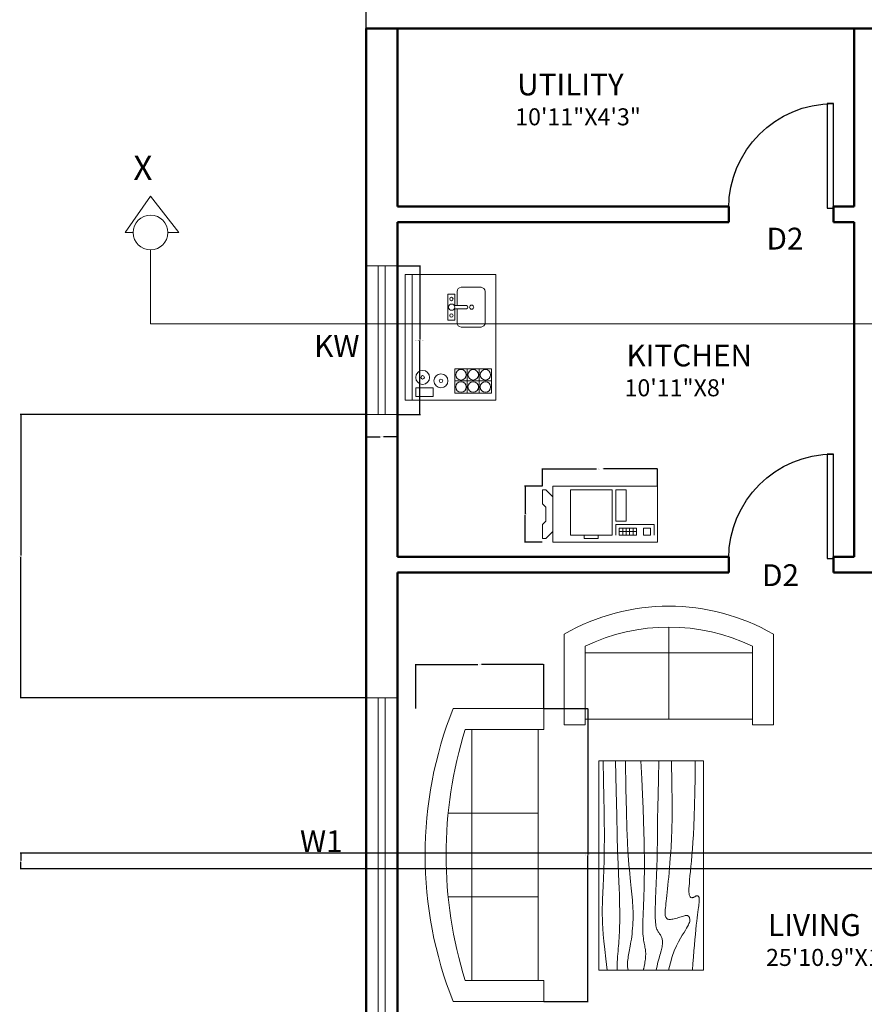
# Model space of a CAD drawing. Units: inches. Extents: x 7359 to 7979, y 33027 to 34263.
# Tile 5 of 32: x 7369 to 7612, y 33347 to 33630. Entities that reach past the tile are written whole.
import ezdxf

# ---------------------------------------------------------------- set-up
doc = ezdxf.new("R2010")
doc.units = ezdxf.units.IN
for name, color, linetype, lineweight in [('A-ANNO-DIMS', 2, 'Continuous', 18), ('A-ANNO-SYMB', 7, 'Continuous', 18), ('A-ANNO-TEXT', 3, 'Continuous', 18), ('A-AREA-IDEN', 7, 'Continuous', 18), ('A-DOOR', 3, 'Continuous', 25), ('A-EQPM', 8, 'Continuous', 18), ('A-FLOR-FIXT', 9, 'Continuous', 18), ('A-FURN', 8, 'Continuous', 18), ('A-GLAZ', 4, 'Continuous', 18), ('A-WALL', 7, 'Continuous', 50)]:
    doc.layers.add(name, color=color, linetype=linetype, lineweight=lineweight)
doc.styles.get("Standard").update_dxf_attribs({"font": 'arial.ttf'})
doc.dimstyles.get("Standard").update_dxf_attribs({"dimtxt": 0.18, "dimasz": 0.18, "dimexe": 0.18, "dimexo": 0.0625, "dimgap": 0.09, "dimtad": 0, "dimtih": 1, "dimtoh": 1, "dimdec": 4, "dimzin": 0, "dimdsep": 46, "dimtxsty": 'Standard', "dimcen": 0.09, "dimadec": 0, "dimazin": 0, "dimtfac": 1, "dimtdec": 4, "dimtofl": 0, "dimtmove": 0, "dimatfit": 3, "dimfxl": 1, "dimtolj": 1, "dimtzin": 0, "dimarcsym": 0})

# ---------------------------------------------------------------- blocks, each defined once
blk = doc.blocks.new('*U2')
for p, q in [((0, 0), (0, -100)), ((750, 0), (750, -100))]:
    blk.add_line(p, q)
blk.add_lwpolyline([(0, 0), (0, 750), (43.75, 750), (43.75, 0)], close=True)
blk.add_arc((0, 0), 750, 0, 90)
blk = doc.blocks.new('Table - Rectangular Woodgrain 60 x 30 in.')
for p, q in [((0, 0), (0, -30)), ((60, 0), (0, 0)), ((60, -30), (60, 0)), ((0, -30), (60, -30))]:
    blk.add_line(p, q)
for points in [[(0, -2.4), (4.8155, -2.418), (9.0302, -2.4688), (12.709, -2.5477), (15.9167, -2.65), (18.7181, -2.7711), (21.1781, -2.9063), (23.3616, -3.0508), (25.3333, -3.2), (27.1477, -3.3495), (28.8172, -3.4958), (30.3437, -3.636), (31.7291, -3.7667), (32.9756, -3.8849), (34.0849, -3.9875), (35.059, -4.0714), (35.9, -4.1334), (36.6114, -4.1711), (37.2041, -4.1854), (37.6906, -4.1779), (38.0833, -4.15), (38.3948, -4.1034), (38.6375, -4.0396), (38.8239, -3.9602), (38.9666, -3.8667), (39.0764, -3.7608), (39.1573, -3.6448), (39.2116, -3.521), (39.2416, -3.3917), (39.2498, -3.2593), (39.2385, -3.1261), (39.21, -2.9944), (39.1666, -2.8667), (39.111, -2.7447), (39.0468, -2.6281), (38.978, -2.5163), (38.9083, -2.4083), (38.8418, -2.3035), (38.7823, -2.201), (38.7337, -2.1001), (38.7, -2), (38.6844, -1.9003), (38.6875, -1.8021), (38.7094, -1.707), (38.75, -1.6167), (38.8094, -1.5326), (38.8875, -1.4563), (38.9844, -1.3893), (39.1, -1.3333), (39.2351, -1.2896), (39.3937, -1.2583), (39.5804, -1.2396), (39.8, -1.2333), (40.057, -1.2396), (40.3562, -1.2583), (40.7023, -1.2896), (41.1, -1.3333), (41.5547, -1.3895), (42.0755, -1.4573), (42.6721, -1.5361), (43.3542, -1.625), (44.1316, -1.7233), (45.014, -1.8302), (46.0114, -1.9449), (47.1333, -2.0667), (48.3862, -2.1947), (49.7625, -2.3281), (51.2513, -2.4663), (52.8416, -2.6083), (54.5226, -2.7535), (56.2833, -2.9011), (58.1127, -3.0501), (60, -3.2)], [(0, -9.2), (6.5759, -9.0858), (11.9385, -9.0365), (16.2527, -9.0418), (19.6833, -9.0917), (22.3952, -9.1759), (24.5531, -9.2844), (26.322, -9.4069), (27.8666, -9.5333), (29.3241, -9.6553), (30.7203, -9.7719), (32.0532, -9.8837), (33.3208, -9.9917), (34.5213, -10.0965), (35.6526, -10.199), (36.7128, -10.2999), (37.7, -10.4), (38.6129, -10.4996), (39.4531, -10.5969), (40.223, -10.6895), (40.925, -10.775), (41.5613, -10.8512), (42.1344, -10.9156), (42.6465, -10.966), (43.1, -11), (43.4976, -11.0158), (43.8437, -11.0136), (44.143, -10.9942), (44.4, -10.9583), (44.6195, -10.9069), (44.8062, -10.8406), (44.9648, -10.7603), (45.1, -10.6667), (45.2155, -10.5598), (45.3114, -10.4365), (45.3871, -10.2929), (45.4416, -10.125), (45.4743, -9.929), (45.4844, -9.7011), (45.4709, -9.4371), (45.4333, -9.1333), (45.3716, -8.7883), (45.2896, -8.4104), (45.1919, -8.0107), (45.0833, -7.6), (44.9685, -7.1893), (44.8521, -6.7896), (44.7388, -6.4117), (44.6333, -6.0667), (44.54, -5.7628), (44.4614, -5.4979), (44.4001, -5.2675), (44.3583, -5.0667), (44.3384, -4.8909), (44.3427, -4.7354), (44.3736, -4.5956), (44.4333, -4.4667), (44.5236, -4.3453), (44.6427, -4.2333), (44.7884, -4.1339), (44.9583, -4.05), (45.1501, -3.9849), (45.3614, -3.9417), (45.59, -3.9234), (45.8333, -3.9333), (46.0915, -3.9749), (46.3734, -4.0531), (46.6906, -4.1736), (47.0542, -4.3417), (47.4756, -4.5629), (47.9661, -4.8427), (48.5372, -5.1866), (49.2, -5.6), (49.9676, -6.0844), (50.8594, -6.625), (51.8965, -7.2031), (53.1, -7.8), (54.491, -8.3969), (56.0906, -8.975), (57.9199, -9.5156), (60, -10)], [(0, -12.8), (5.1847, -12.9322), (9.6213, -13.0323), (13.3963, -13.1059), (16.5958, -13.1583), (19.3063, -13.1952), (21.614, -13.2219), (23.6054, -13.2439), (25.3666, -13.2667), (26.9728, -13.2947), (28.4531, -13.3281), (29.8256, -13.3663), (31.1083, -13.4083), (32.3191, -13.4535), (33.476, -13.501), (34.597, -13.5501), (35.7, -13.6), (36.7984, -13.6497), (37.8875, -13.6979), (38.9578, -13.743), (40, -13.7833), (41.0047, -13.8174), (41.9625, -13.8438), (42.864, -13.8607), (43.7, -13.8667), (44.4631, -13.8604), (45.1552, -13.8417), (45.7801, -13.8104), (46.3416, -13.7667), (46.8439, -13.7104), (47.2906, -13.6417), (47.6858, -13.5604), (48.0333, -13.4667), (48.3375, -13.3608), (48.6042, -13.2448), (48.8396, -13.121), (49.05, -12.9917), (49.2417, -12.8593), (49.4208, -12.7261), (49.5937, -12.5944), (49.7667, -12.4667), (49.9452, -12.3451), (50.1323, -12.2313), (50.3303, -12.1268), (50.5416, -12.0333), (50.7686, -11.9524), (51.0135, -11.8854), (51.2788, -11.8341), (51.5666, -11.8), (51.8785, -11.7843), (52.2116, -11.7865), (52.562, -11.8059), (52.926, -11.8417), (53.2998, -11.8931), (53.6795, -11.9594), (54.0614, -12.0397), (54.4416, -12.1333), (54.8223, -12.2401), (55.2293, -12.3625), (55.6942, -12.5037), (56.2489, -12.6667), (56.9251, -12.8547), (57.7545, -13.0708), (58.7689, -13.3182), (60, -13.6)], [(0, -18), (5.124, -17.7273), (9.6609, -17.5057), (13.6705, -17.3303), (17.2125, -17.1958), (20.3467, -17.0973), (23.1328, -17.0297), (25.6307, -16.9878), (27.9, -16.9667), (29.9928, -16.9617), (31.9302, -16.9703), (33.7254, -16.9907), (35.3917, -17.0208), (36.9423, -17.0588), (38.3906, -17.1026), (39.7499, -17.1503), (41.0333, -17.2), (42.2519, -17.2496), (43.4073, -17.2969), (44.4986, -17.3395), (45.525, -17.375), (46.4858, -17.4012), (47.3802, -17.4156), (48.2074, -17.416), (48.9667, -17.4), (49.6583, -17.3662), (50.2872, -17.3167), (50.8595, -17.2547), (51.3812, -17.1833), (51.8584, -17.1057), (52.2971, -17.025), (52.7034, -16.9443), (53.0833, -16.8667), (53.443, -16.7951), (53.789, -16.7313), (54.128, -16.6768), (54.4666, -16.6334), (54.8115, -16.6024), (55.1693, -16.5854), (55.5465, -16.5841), (55.95, -16.6), (56.3828, -16.6337), (56.8346, -16.6823), (57.2915, -16.7418), (57.7396, -16.8084), (58.165, -16.878), (58.5539, -16.9469), (58.8924, -17.0111), (59.1666, -17.0667), (59.3679, -17.1107), (59.5078, -17.1438), (59.6032, -17.1675), (59.6708, -17.1833), (59.7275, -17.193), (59.7901, -17.1979), (59.8753, -17.1998), (60, -17.2)], [(0, -22.4), (8.0098, -22.2501), (14.4094, -22.1011), (19.4168, -21.9535), (23.25, -21.8083), (26.1269, -21.6663), (28.2656, -21.5281), (29.884, -21.3947), (31.2, -21.2667), (32.3967, -21.1448), (33.5172, -21.0292), (34.5697, -20.9198), (35.5625, -20.8167), (36.5037, -20.7198), (37.4015, -20.6292), (38.2642, -20.5448), (39.1, -20.4667), (39.9164, -20.3951), (40.7187, -20.3313), (41.5117, -20.2768), (42.3, -20.2333), (43.0883, -20.2024), (43.8812, -20.1854), (44.6836, -20.1841), (45.5, -20.2), (46.3328, -20.234), (47.1747, -20.2844), (48.0163, -20.3488), (48.8479, -20.425), (49.66, -20.5106), (50.4429, -20.6031), (51.1872, -20.7004), (51.8833, -20.8), (52.5246, -20.8999), (53.1166, -20.9995), (53.6681, -21.0983), (54.1875, -21.1958), (54.6834, -21.2919), (55.1646, -21.3859), (55.6394, -21.4777), (56.1167, -21.5667), (56.6028, -21.6515), (57.0961, -21.7266), (57.5929, -21.7852), (58.0896, -21.8208), (58.5823, -21.8268), (59.0674, -21.7964), (59.5412, -21.723), (60, -21.6)], [(0, -25.2), (8.6355, -25.0504), (15.7026, -24.9031), (21.4049, -24.7606), (25.9458, -24.625), (29.529, -24.4988), (32.3578, -24.3844), (34.6359, -24.284), (36.5667, -24.2), (38.3213, -24.1341), (39.9417, -24.0854), (41.437, -24.0523), (42.8167, -24.0333), (44.0901, -24.0268), (45.2667, -24.0313), (46.3557, -24.0451), (47.3667, -24.0667), (48.309, -24.0947), (49.1928, -24.1287), (50.0284, -24.168), (50.826, -24.2125), (51.5959, -24.2617), (52.3483, -24.3151), (53.0935, -24.3725), (53.8417, -24.4334), (54.6009, -24.497), (55.3699, -24.561), (56.1454, -24.6226), (56.9239, -24.6792), (57.7021, -24.7279), (58.4764, -24.7662), (59.2435, -24.7911), (60, -24.8)], [(0, -28.8), (5.6867, -28.6681), (10.45, -28.5698), (14.407, -28.5012), (17.675, -28.4584), (20.3711, -28.4374), (22.6125, -28.4344), (24.5164, -28.4455), (26.2, -28.4667), (27.762, -28.4947), (29.2276, -28.5281), (30.6033, -28.5663), (31.8958, -28.6084), (33.1118, -28.6535), (34.2578, -28.7011), (35.3405, -28.7501), (36.3666, -28.8), (37.3443, -28.8497), (38.288, -28.8974), (39.2137, -28.9412), (40.1375, -28.9792), (41.0753, -29.0093), (42.0432, -29.0297), (43.0572, -29.0384), (44.1333, -29.0333), (45.2936, -29.0114), (46.5843, -28.9641), (48.0579, -28.8816), (49.7666, -28.7542), (51.7629, -28.5721), (54.0989, -28.3255), (56.8272, -28.0048), (60, -27.6)]]:
    blk.add_lwpolyline(points)
blk = doc.blocks.new('Sofa - Roundback 7 ft.')
for p, q in [((-12.00002, -32.4421), (-12.00003, -6.5971)), ((11.99997, -32.4421), (11.99998, -6.5971)), ((-36.000027, -34), (-36.000027, -11.4696)), ((-35.999844, -13.3819), (35.9998, -13.3819)), ((35.99998, -34), (35.99998, -11.4696)), ((-36.000027, -32.4421), (35.99998, -32.4421))]:
    blk.add_line(p, q)
for points in [[(-36.000027, -34), (-42.000027, -34), (-42.000027, -8)], [(41.99998, -8), (41.99998, -34), (35.99998, -34)]]:
    blk.add_lwpolyline(points)
for centre, radius, start, end in [((0, -114.25), 114.25, 68.43141, 111.5686), ((-0.00001, -127.1968), 121.1968, 72.72033, 107.2797)]:
    blk.add_arc(centre, radius, start, end)
blk = doc.blocks.new('Sofa - Roundback Loveseat 5 ft.')
for p, q in [((0, -32.44198), (0, -5.99998)), ((-24, -33.99998), (-24, -11.46958)), ((-23.9998, -13.38178), (23.99986, -13.38178)), ((24.00004, -33.99998), (24.00004, -11.46958)), ((-24, -32.44198), (24.00004, -32.44198))]:
    blk.add_line(p, q)
for points in [[(-24, -33.99998), (-30, -33.99998), (-30, -7.99998)], [(30.00004, -7.99998), (30.00004, -33.99998), (24.00004, -33.99998)]]:
    blk.add_lwpolyline(points)
for centre, radius, start, end in [((0, -60.24998), 60.24998, 60.13715, 119.8628), ((0, -61.38438), 55.38444, 64.32083, 115.6792)]:
    blk.add_arc(centre, radius, start, end)
blk = doc.blocks.new('Wet Bar')
for p, q in [((0, 0), (36, 0)), ((0, -26), (0, 0)), ((36, 0), (36, -26)), ((0, -2), (36, -2)), ((3.5, -3), (1, -3)), ((1, -3), (1, -8)), ((3.5, -8), (3.5, -3)), ((1, -8), (3.5, -8)), ((2, -14.25), (9, -14.25)), ((2, -24.75), (2, -14.25)), ((5.5, -14.25), (5.5, -24.75)), ((9, -14.25), (9, -24.75)), ((26.2, -17.55), (26.2, -14.1284)), ((27.1001, -17.55), (27.1001, -14.1284)), ((2, -17.75), (9, -17.75)), ((9, -21.25), (2, -21.25)), ((9, -24.75), (2, -24.75)), ((36, -26), (0, -26))]:
    blk.add_line(p, q)
for points in [[(26.2, -14.25), (22.95, -14.25), (22.95, -12.2), (26.75, -12.2)], [(26.7487, -12.2), (30.3501, -12.2), (30.3501, -14.25), (27.1001, -14.25)], [(20.95, -21.75), (20.95, -16.05)], [(22.15, -14.85), (26.2, -14.85)], [(27.1001, -14.85), (31.15, -14.85)], [(32.3501, -16.05), (32.3501, -21.75)], [(31.15, -22.95), (22.15, -22.95)]]:
    blk.add_lwpolyline(points)
for centre, radius in [((6.5, -5), 2), ((6.5, -5), 0.5), ((5.5, -10.25), 2), ((5.5, -10.25), 0.5), ((24.25, -13.25), 0.5), ((26.65, -13.35), 0.9), ((29, -13.25), 0.5), ((3.75, -16), 1.5), ((7.25, -16), 1.5), ((3.75, -19.5), 1.5), ((7.25, -19.5), 1.5), ((26.65, -19.05), 0.6), ((3.75, -23), 1.5), ((7.25, -23), 1.5)]:
    blk.add_circle(centre, radius)
for centre, radius, start, end in [((22.2251, -16.125), 1.2772, 93.36646, 176.6335), ((31.075, -16.125), 1.2772, 3.366461, 86.63354), ((26.65, -17.55), 0.45, 180, 0), ((22.2251, -21.675), 1.2772, 183.3665, 266.6335), ((31.075, -21.675), 1.2772, 273.3665, 356.6335)]:
    blk.add_arc(centre, radius, start, end)
blk = doc.blocks.new('Copy Machine')
for p, q in [((0, 0), (0, -16)), ((30, 0), (0, 0)), ((30, -16), (30, 0)), ((-3, -1), (-3, -5)), ((-2, -1), (-3, -1)), ((0, -3), (-2, -1)), ((5, -1), (5, -14)), ((17, -1), (5, -1)), ((17, -14), (17, -1)), ((18, -1), (18, -10)), ((21, -1), (18, -1)), ((21, -10), (21, -1)), ((-3, -5), (-2, -6)), ((-2, -10), (-2, -6)), ((-3, -11), (-2, -10)), ((-3, -15), (-3, -11)), ((18, -10), (21, -10)), ((18, -14), (18, -11)), ((18, -11), (29, -11)), ((29, -11), (29, -14)), ((0, -13), (-2, -15)), ((5, -14), (17, -14)), ((9, -14), (9, -15)), ((13, -15), (13, -14)), ((24, -12), (19, -12)), ((19, -12), (19, -14)), ((24, -13), (19, -13)), ((19, -14), (24, -14)), ((20, -12), (20, -14)), ((21, -14), (21, -12)), ((22, -12), (22, -14)), ((23, -14), (23, -12)), ((24, -14), (24, -12)), ((28, -12), (26, -12)), ((26, -12), (26, -14)), ((26, -14), (28, -14)), ((28, -14), (28, -12)), ((-2, -15), (-3, -15)), ((0, -16), (30, -16)), ((9, -15), (13, -15))]:
    blk.add_line(p, q)
blk = doc.blocks.new('SECTION-HEAD')
for p, q in [((0, 4.98), (7.32, 15.43)), ((7.32, 15.43), (15.39, 4.98)), ((2.34, 4.98), (0, 4.98)), ((12.3, 4.98), (15.39, 4.98))]:
    blk.add_line(p, q)
blk.add_circle((7.32, 4.98), 4.98)
blk = doc.blocks.new('WINDOW-W1-LIVING')
for p, q in [((0, 91.75), (9, 91.75)), ((3.5, 0), (3.5, 91.75)), ((5.5, 0), (5.5, 91.75)), ((0, 0), (9, 0))]:
    blk.add_line(p, q)
blk = doc.blocks.new('WINDOW-KW')
for p, q in [((0, 42.66), (9, 42.66)), ((3.5, 42.66), (3.5, 0)), ((5.5, 42.66), (5.5, 0)), ((5.5, 42.66), (5.5, 0)), ((0, 0), (9, 0))]:
    blk.add_line(p, q)
blk = doc.blocks.new('*D40')
at = {"layer": 'A-ANNO-DIMS', "color": 0, "lineweight": -2, "transparency": 16777216}
for p, q in [((7519.73, 33432.15), (7532.45, 33432.15)), ((7532.27, 33431.97), (7532.27, 33390.34)), ((7532.27, 33348.33), (7532.27, 33389.97)), ((7519.73, 33348.15), (7532.45, 33348.15))]:
    blk.add_line(p, q, dxfattribs=at)
at = {"layer": 'A-ANNO-DIMS', "color": 0, "transparency": 16777216}
for points in [[(7532.24, 33431.97), (7532.3, 33431.97), (7532.27, 33432.15)], [(7532.24, 33348.33), (7532.3, 33348.33), (7532.27, 33348.15)]]:
    blk.add_solid(points, dxfattribs=at)
at = {"layer": 'Defpoints', "color": 0, "transparency": 16777216}
for p in [(7519.67, 33432.15), (7532.27, 33432.15), (7519.67, 33348.15)]:
    blk.add_point(p, dxfattribs=at)
at = {"layer": 'A-ANNO-DIMS', "color": 0, "transparency": 16777216, "insert": (7532.27, 33390.15), "char_height": 0.18, "attachment_point": 5}
blk.add_mtext('\\A1;SOFA 84 TYP.', dxfattribs=at)
blk = doc.blocks.new('*D41')
at = {"layer": 'A-ANNO-DIMS', "color": 0, "lineweight": -2, "transparency": 16777216}
for p, q in [((7483.01, 33432.22), (7483.01, 33444.93)), ((7483.19, 33444.75), (7500.81, 33444.75)), ((7519.49, 33444.75), (7501.87, 33444.75)), ((7519.67, 33432.22), (7519.67, 33444.93))]:
    blk.add_line(p, q, dxfattribs=at)
at = {"layer": 'A-ANNO-DIMS', "color": 0, "transparency": 16777216}
for points in [[(7483.19, 33444.78), (7483.19, 33444.72), (7483.01, 33444.75)], [(7519.49, 33444.78), (7519.49, 33444.72), (7519.67, 33444.75)]]:
    blk.add_solid(points, dxfattribs=at)
at = {"layer": 'Defpoints', "color": 0, "transparency": 16777216}
for p in [(7483.01, 33444.75), (7483.01, 33432.15), (7519.67, 33432.15)]:
    blk.add_point(p, dxfattribs=at)
at = {"layer": 'A-ANNO-DIMS', "color": 0, "transparency": 16777216, "insert": (7501.34, 33444.75), "char_height": 0.18, "attachment_point": 5}
blk.add_mtext('\\A1;37 TYP.', dxfattribs=at)
blk = doc.blocks.new('*D44')
at = {"layer": 'A-ANNO-DIMS', "color": 0, "lineweight": -2, "transparency": 16777216}
for p, q in [((7519.31, 33495.98), (7519.31, 33501.05)), ((7519.49, 33500.87), (7534.76, 33500.87)), ((7552.13, 33500.87), (7536.85, 33500.87)), ((7552.31, 33495.98), (7552.31, 33501.05))]:
    blk.add_line(p, q, dxfattribs=at)
at = {"layer": 'A-ANNO-DIMS', "color": 0, "transparency": 16777216}
for points in [[(7519.49, 33500.9), (7519.49, 33500.84), (7519.31, 33500.87)], [(7552.13, 33500.9), (7552.13, 33500.84), (7552.31, 33500.87)]]:
    blk.add_solid(points, dxfattribs=at)
at = {"layer": 'Defpoints', "color": 0, "transparency": 16777216}
for p in [(7552.31, 33500.87), (7519.31, 33495.92), (7552.31, 33495.92)]:
    blk.add_point(p, dxfattribs=at)
at = {"layer": 'A-ANNO-DIMS', "color": 0, "transparency": 16777216, "insert": (7535.81, 33500.87), "char_height": 0.18, "attachment_point": 5}
blk.add_mtext('\\A1;COPIER 33 TYP.', dxfattribs=at)
blk = doc.blocks.new('*D45')
at = {"layer": 'A-ANNO-DIMS', "color": 0, "lineweight": -2, "transparency": 16777216}
for p, q in [((7519.25, 33495.92), (7514.18, 33495.92)), ((7514.36, 33495.74), (7514.36, 33488.1)), ((7514.36, 33480.1), (7514.36, 33487.74)), ((7519.25, 33479.92), (7514.18, 33479.92))]:
    blk.add_line(p, q, dxfattribs=at)
at = {"layer": 'A-ANNO-DIMS', "color": 0, "transparency": 16777216}
for points in [[(7514.33, 33495.74), (7514.39, 33495.74), (7514.36, 33495.92)], [(7514.33, 33480.1), (7514.39, 33480.1), (7514.36, 33479.92)]]:
    blk.add_solid(points, dxfattribs=at)
at = {"layer": 'Defpoints', "color": 0, "transparency": 16777216}
for p in [(7514.36, 33495.92), (7519.31, 33495.92), (7519.31, 33479.92)]:
    blk.add_point(p, dxfattribs=at)
at = {"layer": 'A-ANNO-DIMS', "color": 0, "transparency": 16777216, "insert": (7514.36, 33487.92), "char_height": 0.18, "attachment_point": 5}
blk.add_mtext('\\A1;16 TYP.', dxfattribs=at)
blk = doc.blocks.new('*D58')
at = {"layer": 'A-ANNO-DIMS', "color": 0, "lineweight": -2, "transparency": 16777216}
for p, q in [((7477.79, 33559.14), (7484.31, 33559.14)), ((7484.13, 33558.96), (7484.13, 33538)), ((7484.13, 33516.66), (7484.13, 33537.63)), ((7477.79, 33516.48), (7484.31, 33516.48))]:
    blk.add_line(p, q, dxfattribs=at)
at = {"layer": 'A-ANNO-DIMS', "color": 0, "transparency": 16777216}
for points in [[(7484.1, 33558.96), (7484.16, 33558.96), (7484.13, 33559.14)], [(7484.1, 33516.66), (7484.16, 33516.66), (7484.13, 33516.48)]]:
    blk.add_solid(points, dxfattribs=at)
at = {"layer": 'Defpoints', "color": 0, "transparency": 16777216}
for p in [(7477.73, 33559.14), (7484.13, 33559.14), (7477.73, 33516.48)]:
    blk.add_point(p, dxfattribs=at)
at = {"layer": 'A-ANNO-DIMS', "color": 0, "transparency": 16777216, "insert": (7484.13, 33537.81), "char_height": 0.18, "attachment_point": 5}
blk.add_mtext('\\A1;KITCHEN KW 43 TYP.', dxfattribs=at)
blk = doc.blocks.new('*D59')
at = {"layer": 'A-ANNO-DIMS', "color": 0, "lineweight": -2, "transparency": 16777216}
for p, q in [((7468.73, 33516.42), (7468.73, 33509.91)), ((7477.73, 33516.42), (7477.73, 33509.91)), ((7468.91, 33510.09), (7472.77, 33510.09)), ((7477.55, 33510.09), (7473.68, 33510.09))]:
    blk.add_line(p, q, dxfattribs=at)
at = {"layer": 'A-ANNO-DIMS', "color": 0, "transparency": 16777216}
for points in [[(7468.91, 33510.12), (7468.91, 33510.06), (7468.73, 33510.09)], [(7477.55, 33510.12), (7477.55, 33510.06), (7477.73, 33510.09)]]:
    blk.add_solid(points, dxfattribs=at)
at = {"layer": 'Defpoints', "color": 0, "transparency": 16777216}
for p in [(7468.73, 33516.48), (7477.73, 33516.48), (7477.73, 33510.09)]:
    blk.add_point(p, dxfattribs=at)
at = {"layer": 'A-ANNO-DIMS', "color": 0, "transparency": 16777216, "insert": (7473.23, 33510.09), "char_height": 0.18, "attachment_point": 5}
blk.add_mtext('\\A1;9 TYP.', dxfattribs=at)
blk = doc.blocks.new('*D66')
at = {"layer": 'A-ANNO-DIMS', "color": 0, "lineweight": -2, "transparency": 16777216}
for p, q in [((7468.73, 33627.22), (7468.73, 33657.24)), ((7468.91, 33657.06), (7681.03, 33657.06)), ((7893.95, 33657.06), (7681.82, 33657.06)), ((7894.13, 33627.22), (7894.13, 33657.24))]:
    blk.add_line(p, q, dxfattribs=at)
at = {"layer": 'A-ANNO-DIMS', "color": 0, "transparency": 16777216}
for points in [[(7468.91, 33657.09), (7468.91, 33657.03), (7468.73, 33657.06)], [(7893.95, 33657.09), (7893.95, 33657.03), (7894.13, 33657.06)]]:
    blk.add_solid(points, dxfattribs=at)
at = {"layer": 'Defpoints', "color": 0, "transparency": 16777216}
for p in [(7894.13, 33657.06), (7468.73, 33627.16), (7894.13, 33627.16)]:
    blk.add_point(p, dxfattribs=at)
at = {"layer": 'A-ANNO-DIMS', "color": 0, "transparency": 16777216, "insert": (7681.43, 33657.06), "char_height": 0.18, "attachment_point": 5}
blk.add_mtext('\\A1;425.4', dxfattribs=at)
blk = doc.blocks.new('*D81')
at = {"layer": 'A-ANNO-DIMS', "color": 0, "lineweight": -2, "transparency": 16777216}
for p, q in [((7468.66, 33516.48), (7369.54, 33516.48)), ((7369.72, 33516.3), (7369.72, 33476.05)), ((7369.72, 33435.44), (7369.72, 33475.69)), ((7468.66, 33435.26), (7369.54, 33435.26))]:
    blk.add_line(p, q, dxfattribs=at)
at = {"layer": 'A-ANNO-DIMS', "color": 0, "transparency": 16777216}
for points in [[(7369.69, 33516.3), (7369.75, 33516.3), (7369.72, 33516.48)], [(7369.69, 33435.44), (7369.75, 33435.44), (7369.72, 33435.26)]]:
    blk.add_solid(points, dxfattribs=at)
at = {"layer": 'Defpoints', "color": 0, "transparency": 16777216}
for p in [(7369.72, 33516.48), (7468.73, 33516.48), (7468.73, 33435.26)]:
    blk.add_point(p, dxfattribs=at)
at = {"layer": 'A-ANNO-DIMS', "color": 0, "transparency": 16777216, "insert": (7369.72, 33475.87), "char_height": 0.18, "attachment_point": 5}
blk.add_mtext('\\A1;81.22', dxfattribs=at)
blk = doc.blocks.new('*D85')
at = {"layer": 'A-ANNO-DIMS', "color": 0, "lineweight": -2, "transparency": 16777216}
for p, q in [((7793.06, 33390.66), (7369.54, 33390.66)), ((7369.72, 33390.48), (7369.72, 33388.59)), ((7793.06, 33386.16), (7369.54, 33386.16)), ((7369.72, 33386.34), (7369.72, 33388.23))]:
    blk.add_line(p, q, dxfattribs=at)
at = {"layer": 'A-ANNO-DIMS', "color": 0, "transparency": 16777216}
for points in [[(7369.69, 33390.48), (7369.75, 33390.48), (7369.72, 33390.66)], [(7369.69, 33386.34), (7369.75, 33386.34), (7369.72, 33386.16)]]:
    blk.add_solid(points, dxfattribs=at)
at = {"layer": 'Defpoints', "color": 0, "transparency": 16777216}
for p in [(7793.13, 33390.66), (7369.72, 33386.16), (7793.13, 33386.16)]:
    blk.add_point(p, dxfattribs=at)
at = {"layer": 'A-ANNO-DIMS', "color": 0, "transparency": 16777216, "insert": (7369.72, 33388.41), "char_height": 0.18, "attachment_point": 5}
blk.add_mtext('\\A1;4.5', dxfattribs=at)

msp = doc.modelspace()

# ---------------------------------------------------------------- linework, layer by layer
at = {"layer": 'A-ANNO-SYMB'}
for q in [(7406.9423, 33563.6906), (7940.6696, 33542.482)]:
    msp.add_line((7406.9423, 33542.482), q, dxfattribs=at)
at = {"layer": 'A-WALL'}
for p, q in [((7468.7266, 33627.1623), (7894.1266, 33627.1623)), ((7468.7266, 33627.1623), (7468.7266, 33158.6623)), ((7477.7266, 33627.1623), (7477.7266, 33576.1623)), ((7608.7266, 33627.1623), (7608.7266, 33576.1623)), ((7477.7266, 33576.1623), (7572.7266, 33576.1623)), ((7572.7266, 33576.1623), (7572.7266, 33571.6623)), ((7602.7266, 33576.1623), (7608.7266, 33576.1623)), ((7602.7266, 33576.1623), (7602.7266, 33571.6623)), ((7477.7266, 33571.6623), (7572.7266, 33571.6623)), ((7477.7266, 33571.6623), (7477.7266, 33475.6623)), ((7602.7266, 33571.6623), (7608.7266, 33571.6623)), ((7608.7266, 33571.6623), (7608.7266, 33475.6623)), ((7477.7266, 33475.6623), (7572.7266, 33475.6623)), ((7572.7266, 33475.6623), (7572.7266, 33471.1623)), ((7602.7266, 33475.6623), (7608.7266, 33475.6623)), ((7602.7266, 33475.6623), (7602.7266, 33471.1623)), ((7477.7266, 33471.1623), (7572.7266, 33471.1623)), ((7477.7266, 33471.1623), (7477.7266, 33301.0623)), ((7602.7266, 33471.1623), (7691.2266, 33471.1623))]:
    msp.add_line(p, q, dxfattribs=at)

# ---------------------------------------------------------------- block references
at = {"layer": 'A-ANNO-SYMB'}
msp.add_blockref('SECTION-HEAD', (7399.6221, 33563.6904), dxfattribs=at)
at = {"layer": 'A-DOOR', "xscale": -0.0399999999999999, "yscale": 0.0399999999999999, "zscale": 0.0399999999999999}
for p in [(7602.7266, 33575.6623), (7602.7266, 33475.1623)]:
    msp.add_blockref('*U2', p, dxfattribs=at)
at = {"layer": 'A-EQPM'}
msp.add_blockref('Copy Machine', (7522.3083, 33495.9203), dxfattribs=at)
at = {"layer": 'A-FLOR-FIXT', "rotation": 90}
msp.add_blockref('Wet Bar', (7479.9538, 33520.6382), dxfattribs=at)
at = {"layer": 'A-FURN'}
msp.add_blockref('Sofa - Roundback Loveseat 5 ft.', (7555.532, 33461.52), dxfattribs=at)
for name, p, rotation in [('Sofa - Roundback 7 ft.', (7485.6721, 33390.1541), 90), ('Table - Rectangular Woodgrain 60 x 30 in.', (7565.492, 33417.1564), 270)]:
    msp.add_blockref(name, p, dxfattribs=dict(at, rotation=rotation))
at = {"layer": 'A-GLAZ'}
for name, p in [('WINDOW-KW', (7468.7261, 33516.4844)), ('WINDOW-W1-LIVING', (7468.7261, 33343.5154))]:
    msp.add_blockref(name, p, dxfattribs=at)

# ---------------------------------------------------------------- texts
at = {"layer": 'A-ANNO-SYMB'}
msp.add_text('X', height=6.9459, dxfattribs=at).set_placement((7402.022, 33583.7843))
at = {"layer": 'A-ANNO-TEXT'}
for s, p in [('D2', (7583.5367, 33563.809)), ('KW', (7453.831, 33533.0184)), ('D2', (7582.2569, 33467.2804)), ('W1', (7449.7806, 33390.9721))]:
    msp.add_text(s, height=6.25941, dxfattribs=at).set_placement(p)
at = {"layer": 'A-AREA-IDEN'}
for s, height, p in [('UTILITY', 6.25941, (7512.0433, 33608.0303)), ('10\'11"X4\'3"', 4.885549, (7511.48, 33599.4359)), ('KITCHEN', 6.25941, (7543.3947, 33530.309)), ('10\'11"X8\'', 4.88555, (7542.8315, 33521.7147)), ('LIVING', 6.25941, (7583.9722, 33366.9355)), ('25\'10.9"X14\'1.6"', 4.885549, (7583.409, 33358.3411))]:
    msp.add_text(s, height=height, dxfattribs=at).set_placement(p)

# ---------------------------------------------------------------- dimensions: what is measured, and where the dimension line sits
at = {"layer": 'A-ANNO-DIMS'}
dim = msp.add_linear_dim(base=(7894.1266, 33657.0623), p1=(7468.7266, 33627.1623), p2=(7894.1266, 33627.1623), dimstyle='Standard', override={"dimdec": 1, "dimlfac": 1, "dimrnd": 0, "dimzin": 0, "dimdsep": 46, "dimlunit": 2}, dxfattribs=at)
dim.commit()
dim.dimension.update_dxf_attribs({"geometry": '*D66', "text_midpoint": (7681.4266, 33657.0623)})
for base, p1, p2, angle, text, picture, middle in [((7484.1251, 33559.1413), (7477.7266, 33516.4842), (7477.7266, 33559.1413), 90, 'KITCHEN KW <> TYP.', '*D58', (7484.1251, 33537.8127)), ((7514.3583, 33495.9203), (7519.3083, 33479.9203), (7519.3083, 33495.9203), 90, '<> TYP.', '*D45', (7514.3583, 33487.9203)), ((7483.0054, 33444.7541), (7519.6721, 33432.1541), (7483.0054, 33432.1541), 180, '<> TYP.', '*D41', (7501.3387, 33444.7541)), ((7532.2721, 33432.1541), (7519.6721, 33348.154), (7519.6721, 33432.1541), 90, 'SOFA <> TYP.', '*D40', (7532.2721, 33390.154))]:
    dim = msp.add_linear_dim(base=base, p1=p1, p2=p2, angle=angle, text=text, dimstyle='Standard', override={"dimdec": 0, "dimlfac": 1, "dimrnd": 0, "dimzin": 0, "dimdsep": 46, "dimlunit": 2}, dxfattribs=at)
    dim.commit()
    dim.dimension.update_dxf_attribs({"geometry": picture, "text_midpoint": middle})
for base, p1, p2, override, picture, middle in [((7369.7217, 33516.4842), (7468.7266, 33435.2613), (7468.7266, 33516.4842), {"dimdec": 2, "dimlfac": 1, "dimrnd": 0, "dimzin": 0, "dimdsep": 46, "dimlunit": 2}, '*D81', (7369.7217, 33475.8727)), ((7369.7217, 33386.1623), (7793.1266, 33390.6623), (7793.1266, 33386.1623), {"dimdec": 1, "dimlfac": 1, "dimrnd": 0, "dimzin": 0, "dimdsep": 46, "dimlunit": 2}, '*D85', (7369.7217, 33388.4123))]:
    dim = msp.add_linear_dim(base=base, p1=p1, p2=p2, angle=90, dimstyle='Standard', override=override, dxfattribs=at)
    dim.commit()
    dim.dimension.update_dxf_attribs({"geometry": picture, "text_midpoint": middle})
for base, p1, p2, text, picture, middle in [((7477.7266, 33510.0856), (7468.7266, 33516.4842), (7477.7266, 33516.4842), '<> TYP.', '*D59', (7473.2266, 33510.0856)), ((7552.3083, 33500.8703), (7519.3083, 33495.9203), (7552.3083, 33495.9203), 'COPIER <> TYP.', '*D44', (7535.8083, 33500.8703))]:
    dim = msp.add_linear_dim(base=base, p1=p1, p2=p2, text=text, dimstyle='Standard', override={"dimdec": 0, "dimlfac": 1, "dimrnd": 0, "dimzin": 0, "dimdsep": 46, "dimlunit": 2}, dxfattribs=at)
    dim.commit()
    dim.dimension.update_dxf_attribs({"geometry": picture, "text_midpoint": middle})

doc.saveas('drawing.dxf')
